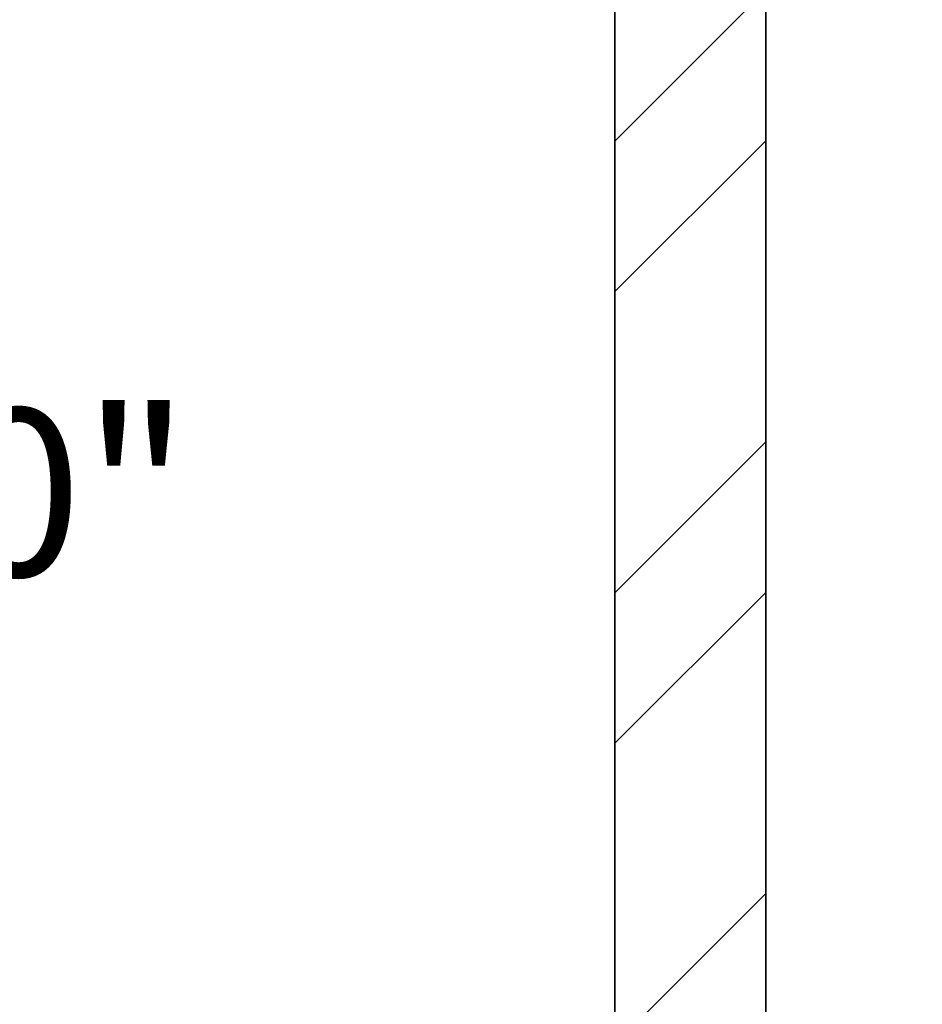
# Model space of a CAD drawing. Units: inches. Extents: x 1885 to 2748, y 783 to 2421.
# Tile 91 of 117: x 2341 to 2368, y 2252 to 2282. Entities that reach past the tile are written whole.
import ezdxf

# ---------------------------------------------------------------- set-up
doc = ezdxf.new("R2010")
doc.units = ezdxf.units.IN
doc.layers.add('A-AREA-IDEN', color=7, linetype='Continuous', lineweight=18)
doc.layers.add('A-WALL', color=7, linetype='Continuous', lineweight=35)
doc.layers.add('A-WALL-PATT', color=85, linetype='Continuous', lineweight=13, true_color=0x58ba48)
doc.styles.get("Standard").update_dxf_attribs({"font": 'arial.ttf'})

msp = doc.modelspace()

# ---------------------------------------------------------------- hatches: boundary and pattern name
at = {"layer": 'A-WALL-PATT'}
h = msp.add_hatch(dxfattribs=at)
h.set_pattern_fill('ANSI32', color=256)
h.paths.add_polyline_path([(2007.772, 2318.006), (1980.774, 2318.006), (1980.774, 2281.215), (1985.274, 2281.215), (1985.274, 2313.506), (2007.772, 2313.506), (2007.772, 2315.756)])
h.paths.add_polyline_path([(2094.324, 2318.006), (2067.772, 2318.006), (2067.772, 2313.506), (2094.324, 2313.506), (2094.324, 2315.756)])
h.paths.add_polyline_path([(2131.367, 2315.756), (2131.367, 2318.006), (2131.189, 2318.006), (2112.609, 2318.006), (2112.609, 2313.506), (2117.274, 2313.506), (2117.274, 2255.201), (2121.774, 2255.201), (2121.774, 2313.506), (2131.367, 2313.506)])
h.paths.add_polyline_path([(2190.512, 2318.006), (2155.367, 2318.006), (2155.367, 2313.506), (2169.774, 2313.506), (2169.774, 2229.506), (2121.774, 2229.506), (2121.774, 2233.451), (2119.524, 2233.451), (2117.274, 2233.451), (2117.274, 2201.101), (2121.774, 2201.101), (2121.774, 2225.006), (2169.774, 2225.006), (2169.774, 2165.006), (2306.274, 2165.006), (2306.274, 2066.006), (2310.774, 2066.006), (2344.274, 2066.006), (2486.274, 2066.006), (2486.274, 1886.006), (2483.02, 1886.006), (2483.02, 1881.506), (2486.274, 1881.506), (2486.274, 1880.678), (2490.774, 1880.678), (2490.774, 2070.506), (2344.274, 2070.506), (2310.774, 2070.506), (2310.774, 2165.006), (2310.774, 2173.636), (2308.524, 2173.636), (2306.274, 2173.636), (2306.274, 2169.506), (2174.274, 2169.506), (2174.274, 2313.506), (2190.512, 2313.506), (2190.512, 2315.756)])
h.paths.add_polyline_path([(1985.274, 2221.215), (1980.774, 2221.215), (1980.774, 2165.006), (1992.774, 2165.006), (1992.774, 2141.927), (1997.274, 2141.927), (1997.274, 2165.006), (2117.274, 2165.006), (2117.274, 2163.126), (2121.774, 2163.126), (2121.774, 2172.734), (2119.524, 2172.734), (2117.274, 2172.734), (2117.274, 2169.506), (1985.274, 2169.506)])
h.paths.add_polyline_path([(1997.274, 2105.927), (1992.774, 2105.927), (1992.774, 2070.506), (2016.774, 2070.506), (2016.774, 2059.123), (2019.024, 2059.123), (2021.274, 2059.123), (2021.274, 2070.506), (2117.274, 2070.506), (2117.274, 2022.506), (2114.423, 2022.506), (2114.423, 2018.006), (2123.627, 2018.006), (2123.627, 2020.256), (2123.627, 2022.506), (2121.774, 2022.506), (2121.774, 2142.587), (2119.524, 2142.587), (2117.274, 2142.587), (2117.274, 2075.006), (1997.274, 2075.006)])
h.paths.add_polyline_path([(2092.029, 2020.256), (2092.029, 2022.506), (2021.274, 2022.506), (2021.274, 2035.123), (2016.774, 2035.123), (2016.774, 2018.006), (2016.774, 1978.784), (2021.274, 1978.784), (2021.274, 2018.006), (2092.029, 2018.006)])
h.paths.add_polyline_path([(2260.938, 2022.506), (2153.105, 2022.506), (2153.105, 2020.256), (2153.105, 2018.006), (2155.274, 2018.006), (2155.274, 1886.006), (2107.629, 1886.006), (2107.629, 1881.506), (2182.911, 1881.506), (2182.911, 1883.756), (2182.911, 1886.006), (2159.774, 1886.006), (2159.774, 2018.006), (2260.938, 2018.006), (2260.938, 2020.256)])
h.paths.add_polyline_path([(2047.629, 1883.756), (2047.629, 1886.006), (2021.274, 1886.006), (2021.274, 1918.784), (2019.024, 1918.784), (2016.774, 1918.784), (2016.774, 1881.506), (2047.629, 1881.506)])
h.paths.add_polyline_path([(2306.361, 1883.756), (2306.361, 1886.006), (2296.274, 1886.006), (2296.274, 1982.006), (2316.535, 1982.006), (2316.535, 1984.256), (2316.535, 1986.506), (2296.274, 1986.506), (2296.274, 2022.506), (2289.276, 2022.506), (2289.276, 2018.006), (2291.774, 2018.006), (2291.774, 1886.006), (2242.911, 1886.006), (2242.911, 1881.506), (2306.361, 1881.506)], flags=17)
h.paths.add_polyline_path([(1985.274, 1843.006), (2021.6, 1843.006), (2021.534, 1845.441), (2021.477, 1847.506), (1980.774, 1847.506), (1980.774, 1809.446), (1985.274, 1809.446)])
h.paths.add_polyline_path([(2131.482, 1845.256), (2131.482, 1847.506), (2081.534, 1847.506), (2081.534, 1843.006), (2117.274, 1843.006), (2117.274, 1784.147), (2119.524, 1784.147), (2121.774, 1784.147), (2121.774, 1843.006), (2131.482, 1843.006)])
h.paths.add_polyline_path([(2203.886, 1847.506), (2155.482, 1847.506), (2155.482, 1843.006), (2169.774, 1843.006), (2169.774, 1759.006), (2121.774, 1759.006), (2121.774, 1761.457), (2117.274, 1761.457), (2117.274, 1730.429), (2121.774, 1730.429), (2121.774, 1754.506), (2177.421, 1754.506), (2177.421, 1756.756), (2177.421, 1759.006), (2174.274, 1759.006), (2174.274, 1843.006), (2203.886, 1843.006)])
h.paths.add_polyline_path([(2335.554, 1845.256), (2335.554, 1847.506), (2239.886, 1847.506), (2239.886, 1843.006), (2306.274, 1843.006), (2306.274, 1759.006), (2199.486, 1759.006), (2199.486, 1754.506), (2310.774, 1754.506), (2310.774, 1843.006), (2335.554, 1843.006)])
h.paths.add_polyline_path([(2348.774, 2022.506), (2344.274, 2022.506), (2344.274, 1986.506), (2341.681, 1986.506), (2341.681, 1982.006), (2344.274, 1982.006), (2344.274, 1886.006), (2330.361, 1886.006), (2330.361, 1881.506), (2361.627, 1881.506), (2361.627, 1883.756), (2361.627, 1886.006), (2348.774, 1886.006)], flags=17)
h.paths.add_polyline_path([(2283.251, 2315.756), (2283.251, 2318.006), (2238.512, 2318.006), (2238.512, 2313.506), (2283.251, 2313.506)], flags=17)
h.paths.add_polyline_path([(2363.274, 2348.006), (2388.677, 2348.006), (2388.677, 2350.256), (2388.677, 2352.506), (2358.774, 2352.506), (2358.774, 2348.006), (2358.774, 2318.006), (2344.481, 2318.006), (2344.481, 2313.506), (2358.774, 2313.506), (2358.774, 2229.506), (2310.774, 2229.506), (2310.774, 2231.952), (2306.274, 2231.952), (2306.274, 2205.611), (2310.774, 2205.611), (2310.774, 2225.006), (2358.774, 2225.006), (2358.774, 2211.506), (2452.329, 2211.506), (2452.329, 2213.756), (2452.329, 2216.006), (2363.274, 2216.006), (2363.274, 2318.006)])
h.paths.add_polyline_path([(2310.774, 2313.506), (2320.481, 2313.506), (2320.481, 2315.756), (2320.481, 2318.006), (2302.728, 2318.006), (2302.728, 2313.506), (2306.274, 2313.506), (2306.274, 2251.076), (2310.774, 2251.076)], flags=17)
h.paths.add_polyline_path([(2490.774, 2352.506), (2486.274, 2352.506), (2448.677, 2352.506), (2448.677, 2348.006), (2486.274, 2348.006), (2486.274, 2318.006), (2486.274, 2216.006), (2481.78, 2216.006), (2481.78, 2211.506), (2486.274, 2211.506), (2486.274, 2165.006), (2493.289, 2165.006), (2493.289, 2167.256), (2493.289, 2169.506), (2490.774, 2169.506), (2490.774, 2313.506), (2494.429, 2313.506), (2494.429, 2318.006), (2490.774, 2318.006)])
h.paths.add_polyline_path([(2534.653, 2318.006), (2515.691, 2318.006), (2515.691, 2313.506), (2534.653, 2313.506), (2534.653, 2315.756)])
h.paths.add_polyline_path([(2618.274, 2318.006), (2594.653, 2318.006), (2594.653, 2313.506), (2613.774, 2313.506), (2613.774, 2281.706), (2618.274, 2281.706)])
h.paths.add_polyline_path([(2618.274, 2221.706), (2613.774, 2221.706), (2613.774, 2169.506), (2554.019, 2169.506), (2554.019, 2165.006), (2613.774, 2165.006), (2613.774, 2152.878), (2618.274, 2152.878)])
h.paths.add_polyline_path([(2618.274, 2128.878), (2616.024, 2128.878), (2613.774, 2128.878), (2613.774, 2117.006), (2529.774, 2117.006), (2529.774, 2165.006), (2532.848, 2165.006), (2532.848, 2169.506), (2522.867, 2169.506), (2522.867, 2165.006), (2525.274, 2165.006), (2525.274, 2117.006), (2525.274, 2112.506), (2525.274, 2108.576), (2529.774, 2108.576), (2529.774, 2112.506), (2613.774, 2112.506), (2613.774, 2080.19), (2618.274, 2080.19)])
h.paths.add_polyline_path([(2618.274, 2044.19), (2616.024, 2044.19), (2613.774, 2044.19), (2613.774, 2015.506), (2529.774, 2015.506), (2529.774, 2088.582), (2527.524, 2088.582), (2525.274, 2088.582), (2525.274, 2011.006), (2613.774, 2011.006), (2613.774, 1956.755), (2618.274, 1956.755)])
h.paths.add_polyline_path([(2618.274, 1881.506), (2618.274, 1896.755), (2613.774, 1896.755), (2613.774, 1881.506), (2613.774, 1847.506), (2592.715, 1847.506), (2592.715, 1843.006), (2613.774, 1843.006), (2613.774, 1765.006), (2613.774, 1760.506), (2609.621, 1760.506), (2609.621, 1756.006), (2613.774, 1756.006), (2613.774, 1660.006), (2608.544, 1660.006), (2608.544, 1655.506), (2613.774, 1655.506), (2613.774, 1508.158), (2618.274, 1508.158)])
h.paths.add_polyline_path([(2565.774, 1843.006), (2568.997, 1843.006), (2568.997, 1847.506), (2490.774, 1847.506), (2490.774, 1849.7), (2488.524, 1849.7), (2486.274, 1849.7), (2486.274, 1847.506), (2477.274, 1847.506), (2477.274, 1838.506), (2477.274, 1821.493), (2486.274, 1821.493), (2486.274, 1838.506), (2561.274, 1838.506), (2561.274, 1765.006), (2486.274, 1765.006), (2486.274, 1786.157), (2477.274, 1786.157), (2477.274, 1765.006), (2477.274, 1756.006), (2486.274, 1756.006), (2565.774, 1756.006), (2585.621, 1756.006), (2585.621, 1758.256), (2585.621, 1760.506), (2565.774, 1760.506), (2565.774, 1765.006)])
h.paths.add_polyline_path([(2486.274, 1651.006), (2561.274, 1651.006), (2561.274, 1567.006), (2486.274, 1567.006), (2486.274, 1591.321), (2477.274, 1591.321), (2477.274, 1567.006), (2477.274, 1558.006), (2477.274, 1555.439), (2481.774, 1555.439), (2481.774, 1558.006), (2568.653, 1558.006), (2568.653, 1560.256), (2568.653, 1562.506), (2565.774, 1562.506), (2565.774, 1655.506), (2584.544, 1655.506), (2584.544, 1657.756), (2584.544, 1660.006), (2565.774, 1660.006), (2486.274, 1660.006), (2477.274, 1660.006), (2477.274, 1651.006), (2477.274, 1632.989), (2486.274, 1632.989)])
h.paths.add_polyline_path([(2449.967, 1883.756), (2449.967, 1886.006), (2421.627, 1886.006), (2421.627, 1881.506), (2449.967, 1881.506)], flags=17)
h.paths.add_polyline_path([(2447.274, 1847.506), (2395.554, 1847.506), (2395.554, 1843.006), (2442.774, 1843.006), (2442.774, 1809.27), (2447.274, 1809.27)])
h.paths.add_polyline_path([(1985.274, 1749.446), (1980.774, 1749.446), (1980.774, 1694.504), (1985.274, 1694.504), (1985.274, 1694.506), (1986.897, 1694.506), (1986.897, 1697.78), (1986.897, 1699.006), (1985.274, 1699.006)])
h.paths.add_polyline_path([(2152.774, 1699.006), (2121.774, 1699.006), (2121.774, 1703.668), (2119.524, 1703.668), (2117.274, 1703.668), (2117.274, 1699.006), (2009.219, 1699.006), (2009.219, 1694.506), (2148.274, 1694.506), (2148.274, 1692.631), (2152.774, 1692.631)])
h.paths.add_polyline_path([(2016.274, 1694.506), (2011.774, 1694.506), (2011.774, 1558.006), (2040.806, 1558.006), (2040.806, 1560.256), (2040.806, 1562.506), (2016.274, 1562.506)])
h.paths.add_polyline_path([(2152.774, 1663.017), (2150.524, 1663.017), (2148.274, 1663.017), (2148.274, 1562.506), (2100.806, 1562.506), (2100.806, 1558.006), (2165.119, 1558.006), (2165.119, 1560.256), (2165.119, 1562.506), (2152.774, 1562.506), (2152.774, 1610.506), (2224.774, 1610.506), (2224.774, 1607.99), (2229.274, 1607.99), (2229.274, 1615.006), (2152.774, 1615.006)])
h.paths.add_polyline_path([(2238.613, 1560.256), (2238.613, 1562.506), (2229.274, 1562.506), (2229.274, 1588.756), (2227.024, 1588.763), (2224.774, 1588.771), (2224.774, 1562.506), (2189.119, 1562.506), (2189.119, 1558.006), (2238.613, 1558.006)])
h.paths.add_polyline_path([(2336.024, 1560.256), (2336.024, 1562.506), (2310.774, 1562.506), (2310.774, 1656.347), (2308.524, 1656.347), (2306.274, 1656.347), (2306.274, 1562.506), (2286.613, 1562.506), (2286.613, 1558.006), (2336.024, 1558.006)])
h.paths.add_polyline_path([(2447.274, 1690.968), (2445.024, 1690.968), (2442.774, 1690.968), (2442.774, 1687.006), (2306.274, 1687.006), (2306.274, 1680.75), (2310.774, 1680.75), (2310.774, 1682.506), (2442.774, 1682.506), (2442.774, 1562.506), (2396.024, 1562.506), (2396.024, 1558.006), (2447.274, 1558.006)])
h.paths.add_polyline_path([(2447.274, 1749.27), (2445.024, 1749.27), (2442.774, 1749.27), (2442.774, 1717.232), (2447.274, 1717.232)])
h.paths.add_polyline_path([(2044.674, 1521.756), (2044.674, 1524.006), (2007.274, 1524.006), (2007.274, 1503.49), (2009.524, 1503.49), (2011.774, 1503.49), (2011.774, 1519.506), (2044.674, 1519.506)])
h.paths.add_polyline_path([(2177.969, 1521.756), (2177.969, 1524.006), (2104.674, 1524.006), (2104.674, 1519.506), (2145.774, 1519.506), (2145.774, 1387.506), (2143.37, 1387.506), (2143.37, 1383.006), (2251.585, 1383.006), (2251.585, 1385.256), (2251.585, 1387.506), (2150.274, 1387.506), (2150.274, 1519.506), (2177.969, 1519.506)])
h.paths.add_polyline_path([(2298.704, 1524.006), (2237.969, 1524.006), (2237.969, 1519.506), (2282.274, 1519.506), (2282.274, 1387.506), (2279.683, 1387.506), (2279.683, 1383.006), (2286.774, 1383.006), (2286.774, 1419.006), (2312.451, 1419.006), (2312.451, 1421.256), (2312.451, 1423.506), (2286.774, 1423.506), (2286.774, 1519.506), (2298.704, 1519.506), (2298.704, 1521.722)], flags=17)
h.paths.add_polyline_path([(2361.897, 1521.756), (2361.897, 1524.006), (2322.704, 1524.006), (2322.704, 1519.506), (2334.774, 1519.506), (2334.774, 1423.506), (2331.93, 1423.506), (2331.93, 1419.006), (2334.774, 1419.006), (2334.774, 1387.506), (2334.774, 1383.228), (2339.274, 1383.228), (2339.274, 1387.506), (2339.274, 1519.506), (2361.897, 1519.506)], flags=17)
h.paths.add_polyline_path([(2447.274, 1521.756), (2447.274, 1524.006), (2421.897, 1524.006), (2421.897, 1519.506), (2447.274, 1519.506)], flags=17)
h.paths.add_polyline_path([(2481.774, 1529.6), (2479.524, 1529.6), (2477.274, 1529.6), (2477.274, 1524.006), (2474.489, 1524.006), (2474.489, 1519.506), (2477.274, 1519.506), (2477.274, 1334.506), (2296.774, 1334.506), (2296.774, 1240.506), (2160.274, 1240.506), (2160.274, 1180.506), (2112.274, 1180.506), (2112.274, 1207.692), (2110.024, 1207.692), (2107.774, 1207.692), (2107.774, 1171.609), (2112.274, 1171.609), (2112.274, 1176.006), (2160.274, 1176.006), (2160.274, 1092.006), (2144.221, 1092.006), (2144.221, 1087.506), (2189.497, 1087.506), (2189.497, 1089.756), (2189.497, 1092.006), (2164.774, 1092.006), (2164.774, 1236.006), (2296.774, 1236.006), (2296.774, 1231.912), (2301.274, 1231.912), (2301.274, 1330.006), (2481.774, 1330.006), (2481.774, 1387.506)])
h.paths.add_polyline_path([(2618.274, 1448.158), (2613.774, 1448.158), (2613.774, 1382.506), (2529.774, 1382.506), (2525.274, 1382.506), (2525.274, 1307.062), (2529.774, 1307.062), (2529.774, 1378.006), (2613.774, 1378.006), (2613.774, 1354.988), (2618.274, 1354.988)])
h.paths.add_polyline_path([(2618.274, 1318.988), (2613.774, 1318.988), (2613.774, 1281.006), (2529.774, 1281.006), (2529.774, 1283.786), (2527.524, 1283.786), (2525.274, 1283.786), (2525.274, 1228.506), (2516.794, 1228.506), (2516.794, 1224.006), (2533.484, 1224.006), (2533.484, 1226.256), (2533.484, 1228.506), (2529.774, 1228.506), (2529.774, 1276.506), (2613.774, 1276.506), (2613.774, 1266.02), (2618.274, 1266.02)])
h.paths.add_polyline_path([(2618.274, 1134.964), (2613.774, 1134.964), (2613.774, 1092.006), (2594.545, 1092.006), (2594.545, 1087.506), (2618.274, 1087.506)])
h.paths.add_polyline_path([(2534.545, 1092.006), (2509.765, 1092.006), (2509.765, 1087.506), (2534.545, 1087.506), (2534.545, 1089.756)])
h.paths.add_polyline_path([(2481.274, 1224.006), (2484.117, 1224.006), (2484.117, 1226.256), (2484.117, 1228.506), (2476.774, 1228.506), (2476.774, 1198.506), (2471.61, 1198.506), (2471.61, 1194.006), (2476.774, 1194.006), (2476.774, 1062.006), (2436.894, 1062.006), (2436.894, 1057.506), (2476.774, 1057.506), (2481.274, 1057.506), (2481.274, 1062.006), (2481.274, 1087.506), (2485.354, 1087.506), (2485.354, 1089.756), (2485.354, 1092.006), (2481.274, 1092.006), (2481.274, 1117.506)])
h.paths.add_polyline_path([(2439.898, 1198.506), (2349.274, 1198.506), (2349.274, 1194.006), (2349.274, 1180.506), (2301.274, 1180.506), (2301.274, 1201.896), (2299.024, 1201.896), (2296.774, 1201.896), (2296.774, 1172.335), (2299.024, 1172.335), (2301.274, 1172.335), (2301.274, 1176.006), (2349.274, 1176.006), (2349.274, 1092.006), (2334.452, 1092.006), (2334.452, 1087.506), (2349.274, 1087.506), (2349.274, 1057.506), (2353.774, 1057.506), (2376.894, 1057.506), (2376.894, 1059.756), (2376.894, 1062.006), (2353.774, 1062.006), (2353.774, 1087.506), (2353.774, 1180.506), (2353.774, 1194.006), (2439.898, 1194.006), (2439.898, 1196.256)])
h.paths.add_polyline_path([(2270.596, 1089.756), (2270.596, 1092.006), (2249.497, 1092.006), (2249.497, 1087.506), (2270.596, 1087.506)], flags=17)
h.paths.add_polyline_path([(2310.452, 1092.006), (2301.274, 1092.006), (2301.274, 1153.292), (2296.774, 1153.292), (2296.774, 1092.006), (2293.786, 1092.006), (2293.786, 1087.506), (2310.452, 1087.506), (2310.452, 1089.756)], flags=17)
h.paths.add_polyline_path([(2112.274, 1150.328), (2110.024, 1150.328), (2107.774, 1150.328), (2107.774, 1092.006), (2104.465, 1092.006), (2104.465, 1087.506), (2120.221, 1087.506), (2120.221, 1089.756), (2120.221, 1092.006), (2112.274, 1092.006)])
h.paths.add_polyline_path([(2082.172, 1092.006), (2058.144, 1092.006), (2058.144, 1087.506), (2082.172, 1087.506), (2082.172, 1089.756)])
h.paths.add_polyline_path([(1975.774, 1145.638), (1971.274, 1145.638), (1971.274, 1087.506), (1980.774, 1087.506), (1998.144, 1087.506), (1998.144, 1089.756), (1998.144, 1092.006), (1985.274, 1092.006), (1975.774, 1092.006)])
h.paths.add_polyline_path([(2112.274, 1244.385), (2110.024, 1244.385), (2107.774, 1244.385), (2107.774, 1240.506), (1992.274, 1240.506), (1992.274, 1271.008), (1987.774, 1271.008), (1987.774, 1240.506), (1980.774, 1240.506), (1975.774, 1240.506), (1971.274, 1240.506), (1971.274, 1205.638), (1975.774, 1205.638), (1975.774, 1236.006), (2107.774, 1236.006), (2107.774, 1233.444), (2112.274, 1233.444), (2112.274, 1236.006)])
h.paths.add_polyline_path([(2112.274, 1383.006), (2114.783, 1383.006), (2114.783, 1385.256), (2114.783, 1387.506), (2102.476, 1387.506), (2102.476, 1383.006), (2107.774, 1383.006), (2107.774, 1335.006), (2011.774, 1335.006), (2011.774, 1349.939), (2007.274, 1349.939), (2007.274, 1335.006), (1987.774, 1335.006), (1987.774, 1330.506), (1987.774, 1307.008), (1992.274, 1307.008), (1992.274, 1330.506), (2007.274, 1330.506), (2107.774, 1330.506), (2107.774, 1264.711), (2112.274, 1264.711)])
h.paths.add_polyline_path([(2077.857, 1387.506), (2011.774, 1387.506), (2011.774, 1390.036), (2009.524, 1390.036), (2007.274, 1390.036), (2007.274, 1373.939), (2011.774, 1373.939), (2011.774, 1383.006), (2077.857, 1383.006)])
h.paths.add_polyline_path([(2011.774, 1443.49), (2007.274, 1443.49), (2007.274, 1410.248), (2011.774, 1410.248)])

# ---------------------------------------------------------------- linework, layer by layer
at = {"layer": 'A-WALL'}
for p, q in [((2363.274, 2318.006), (2363.274, 2216.006)), ((2358.774, 2313.506), (2358.774, 2229.506))]:
    msp.add_line(p, q, dxfattribs=at)

# ---------------------------------------------------------------- texts
at = {"layer": 'A-AREA-IDEN', "insert": (2317.321, 2278.309), "char_height": 5, "attachment_point": 1}
msp.add_mtext_dynamic_manual_height_columns('TOILET\\P4\'0"x7\'0"', width=94.60671, gutter_width=12.5, heights=[0], dxfattribs=at)

doc.saveas('drawing.dxf')
